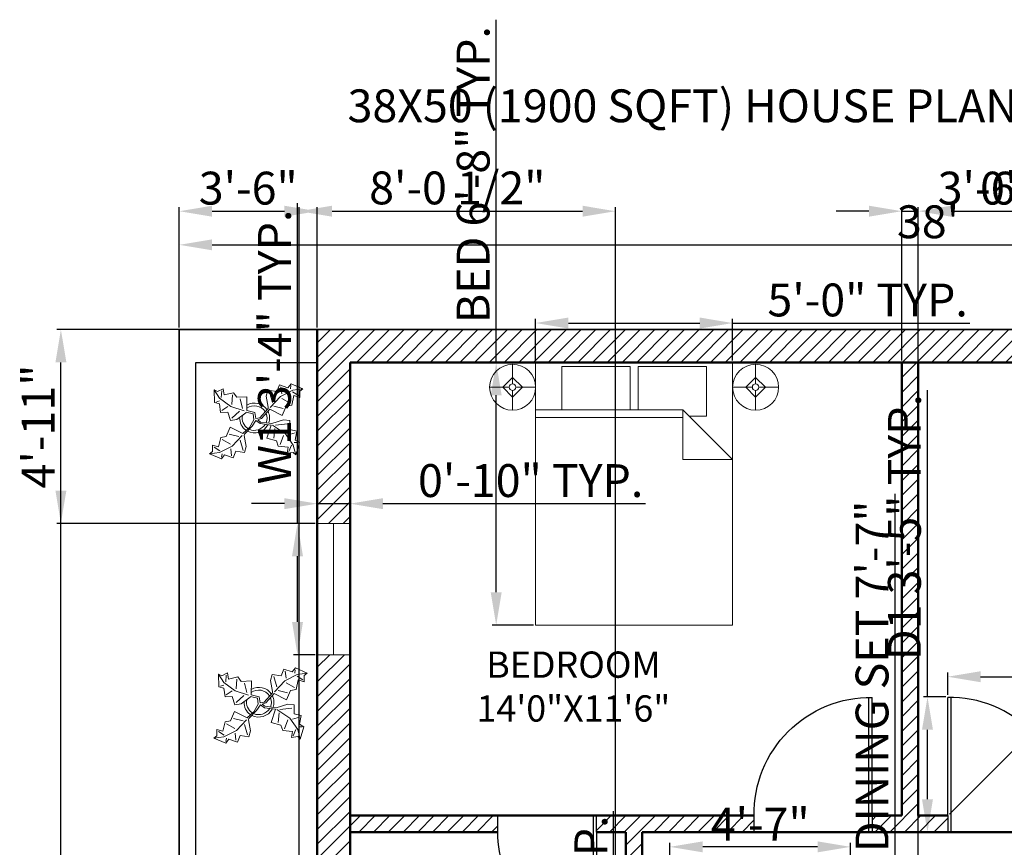
# Model space of a CAD drawing. Units: inches. Extents: x 2206 to 2843, y 1750 to 2489.
# Tile 6 of 8: x 2206 to 2506, y 2237 to 2489. Entities that reach past the tile are written whole.
import ezdxf

# ---------------------------------------------------------------- set-up
doc = ezdxf.new("R2010")
doc.units = ezdxf.units.IN
for name, color, linetype, lineweight in [('A-ANNO-DIMS', 2, 'Continuous', 18), ('A-ANNO-TEXT', 7, 'Continuous', 25), ('A-AREA-IDEN', 7, 'Continuous', 18), ('A-DOOR', 3, 'Continuous', 25), ('A-FURN', 21, 'Continuous', 18), ('A-GLAZ', 4, 'Continuous', 18), ('A-WALL', 7, 'Continuous', 50), ('A-WALL-PATT', 252, 'Continuous', 13), ('C-PROP', 7, 'Continuous', 35), ('L-PLNT', 92, 'Continuous', 18), ('L-SITE-WALL', 8, 'Continuous', 25)]:
    doc.layers.add(name, color=color, linetype=linetype, lineweight=lineweight)
doc.styles.get("Standard").update_dxf_attribs({"font": 'arial.ttf'})
doc.dimstyles.new('ISO-25', dxfattribs={"dimtxt": 10, "dimasz": 10, "dimexe": 1.25, "dimexo": 0.625, "dimtad": 1, "dimdec": 1, "dimlunit": 3, "dimtxsty": 'Standard', "dimcen": 2.5, "dimadec": 0, "dimazin": 0, "dimtfac": 1, "dimtdec": 1, "dimtmove": 0, "dimatfit": 3, "dimfxl": 1, "dimarcsym": 0})

# ---------------------------------------------------------------- blocks, each defined once
blk = doc.blocks.new('Plant - Rubber or Philodendron')
for p, q in [((-14.8639, 10.7964), (-12.6195, 11.8975)), ((-12.6195, 11.8975), (-12.1909, 9.4345)), ((8.8871, 10.7908), (9.9809, 13.4933)), ((9.9809, 13.4933), (13.3837, 12.301)), ((10.5828, 12.6946), (10.8893, 9.7953)), ((13.3837, 12.301), (14.68, 13.9039)), ((14.5816, 13.2037), (14.3848, 11.8033)), ((14.68, 13.9039), (19.3848, 11.8146)), ((-16.2005, 11.4774), (-13.9899, 8.1064)), ((-16.2005, 11.4774), (-14.8639, 10.7964)), ((-16.0159, 6.3329), (-16.2005, 11.4774)), ((-13.9899, 8.1064), (-9.5434, 4.7185)), ((-13.3174, 8.325), (-13.0735, 11.0065)), ((-12.1909, 9.4345), (-8.3829, 10.3)), ((-8.8369, 9.409), (-9.0894, 5.6095)), ((-8.3829, 10.3), (-7.0549, 8.501)), ((-7.0549, 8.501), (-3.0284, 8.6941)), ((-3.0284, 8.6941), (-3.0709, 3.1041)), ((4.6914, 8.8812), (5.3859, 11.2828)), ((4.6914, 8.8812), (5.5014, 4.4831)), ((5.3859, 11.2828), (8.8871, 10.7908)), ((5.9878, 10.4842), (7.1971, 6.3869)), ((10.3916, 8.7942), (6.2847, 4.4028)), ((15.3859, 11.3055), (10.3916, 8.7942)), ((14.2977, 6.1031), (10.9934, 7.9956)), ((15.7909, 9.1065), (14.8995, 5.3044)), ((15.2875, 10.6053), (17.5907, 9.2105)), ((19.3848, 11.8146), (15.3859, 11.3055)), ((18.1925, 8.4119), (15.7909, 9.1065)), ((19.3848, 11.8146), (18.1868, 10.9119)), ((18.1868, 10.9119), (18.1925, 8.4119)), ((-14.0069, 5.8704), (-16.0159, 6.3329)), ((-15.3434, 6.5514), (-13.9984, 6.9884)), ((-13.5868, 2.2894), (-14.0069, 5.8704)), ((-13.1329, 3.1804), (-10.6614, 4.727)), ((-9.5434, 4.7185), (-4.1917, 2.9888)), ((-4.8529, 4.012), (-5.7184, 7.82)), ((5.4346, 3.9146), (5.5014, 4.4831)), ((7.7005, 4.8881), (11.5025, 3.9967)), ((12.7005, 4.8994), (11.1089, 1.1958)), ((14.8995, 5.3044), (12.7005, 4.8994)), ((-10.6784, 2.491), (-13.5868, 2.2894)), ((-9.5858, -0.8715), (-10.6784, 2.491)), ((-9.1318, 0.0195), (-5.9793, 2.9025)), ((-7.1228, -0.443), (-3.5248, 2.2131)), ((-3.5248, 2.2131), (-3.3011, 2.4355)), ((-3.3011, 2.4355), (-0.5306, 1.7947)), ((-3.0709, 3.1041), (0.0797, 2.3163)), ((-0.5306, 1.7947), (-0.2255, -0.5527)), ((-0.5306, 1.7947), (-0.5306, 1.7947)), ((0.0797, 2.3163), (0.4866, -0.031)), ((0.4866, -0.031), (2.1141, 0.2298)), ((2.1141, 0.2298), (5.4346, 3.9146)), ((6.1032, 3.6844), (2.8262, -0.031)), ((11.1089, 1.1958), (6.1032, 3.6844)), ((-11.3237, -7.2629), (-9.7321, -3.5593)), ((-9.7321, -3.5593), (-4.7264, -6.0479)), ((-7.1228, -0.443), (-9.5858, -0.8715)), ((-2.019, -3.6148), (-4.7264, -6.0479)), ((-4.0579, -6.2781), (-0.9375, -3.1608)), ((-2.019, -3.6148), (-0.2255, -0.5527)), ((-0.9375, -3.1608), (0.5883, -0.8135)), ((0.5883, -0.8135), (2.2447, -2.0916)), ((2.8262, -0.031), (1.3003, -0.5527)), ((1.3003, -0.5527), (2.4193, -1.4655)), ((2.2447, -2.0916), (6.7108, -2.6626)), ((2.4193, -1.4655), (6.895, -2.1175)), ((4.943, -7.9659), (6.7108, -2.6626)), ((11.6605, -0.5413), (6.895, -2.1175)), ((12.3677, -6.1981), (7.219, -2.6772)), ((8.3544, -2.7453), (13.1973, -2.1704)), ((11.6605, -0.5413), (14.1354, -0.8948)), ((14.1354, -0.8948), (14.1354, -4.4304)), ((-14.4141, -11.4699), (-13.5228, -7.6679)), ((-13.5228, -7.6679), (-11.3237, -7.2629)), ((-6.3237, -7.2516), (-10.1257, -6.3602)), ((-9.0148, -11.1577), (-4.9047, -6.8122)), ((-4.1246, -6.8466), (-4.0579, -6.2781)), ((-3.3146, -11.2447), (-4.1246, -6.8466)), ((8.125, -4.0768), (7.7715, -7.9659)), ((10.2463, -10.4408), (11.6605, -6.9053)), ((15.5496, -10.7943), (12.3677, -6.1981)), ((16.2567, -5.8446), (13.4283, -6.5517)), ((14.1354, -4.4304), (16.9638, -5.1375)), ((16.9638, -5.1375), (16.2567, -8.673)), ((-16.8157, -10.7754), (-14.4141, -11.4699)), ((-16.8101, -13.2754), (-16.8157, -10.7754)), ((-13.9107, -12.9688), (-16.2139, -11.574)), ((-14.0091, -13.669), (-9.0148, -11.1577)), ((-12.921, -8.4665), (-9.6166, -10.359)), ((-4.611, -12.8477), (-5.8203, -8.7504)), ((-3.3146, -11.2447), (-4.0092, -13.6463)), ((8.8321, -9.0266), (4.943, -7.9659)), ((9.5392, -11.1479), (8.8321, -9.0266)), ((13.4283, -11.5015), (9.5392, -11.1479)), ((13.0748, -13.9763), (13.4283, -11.5015)), ((14.8425, -10.7943), (13.7819, -13.2692)), ((16.6103, -14.6834), (15.5496, -10.7943)), ((17.3174, -9.7337), (15.9032, -9.7337)), ((16.2567, -8.673), (18.0245, -9.7337)), ((18.0245, -9.7337), (16.6103, -14.6834)), ((-18.008, -14.1781), (-16.8101, -13.2754)), ((-18.008, -14.1781), (-14.0091, -13.669)), ((-13.3032, -16.2674), (-18.008, -14.1781)), ((-12.0069, -14.6645), (-13.3032, -16.2674)), ((-13.2048, -15.5672), (-13.008, -14.1668)), ((-8.6042, -15.8568), (-12.0069, -14.6645)), ((-9.206, -15.0581), (-9.5126, -12.1588)), ((-7.5103, -13.1543), (-8.6042, -15.8568)), ((-4.0092, -13.6463), (-7.5103, -13.1543)), ((15.5496, -13.6228), (13.0748, -13.9763)), ((16.6103, -14.6834), (15.5496, -13.6228))]:
    blk.add_line(p, q)
for centre, radius, start, end in [((0, 0), 6.1275, 34.37569, 120.1028), ((-0.0601, -0.2075), 5.2461, 33.82192, 124.9414), ((0.0308, 0.1664), 6, 178.6147, 235.1169), ((0.0308, 0.1664), 5, 168.1647, 238.6725), ((-0.2664, 0.1682), 5.2775, 338.4094, 20.03007), ((-0.098, 0.1364), 6.1288, 341.2017, 26.09184), ((-0.0234, 0.3825), 6.1492, 242.5812, 331.2714), ((-0.1102, 0.4886), 5.2883, 247.3711, 327.472)]:
    blk.add_arc(centre, radius, start, end)
blk = doc.blocks.new('Bed - Queen')
for p, q in [((0, -80.00003), (0, 0)), ((0, 0), (59.99999, 0)), ((59.99999, 0), (59.99999, -80.00003)), ((7.99999, -1.2), (28.79998, -1.2)), ((7.99999, -14.4), (7.99999, -1.2)), ((28.79998, -1.2), (28.79998, -14.4)), ((31.19999, -1.2), (51.99999, -1.2)), ((31.19999, -14.4), (31.19999, -1.2)), ((51.99999, -1.2), (51.99999, -16.4)), ((0, -14.4), (44.8, -14.4)), ((59.99999, -29.6), (44.8, -14.4)), ((44.8, -14.4), (44.8, -29.6)), ((44.8, -16.8), (0, -16.8)), ((51.99999, -16.4), (46.79936, -16.4)), ((44.8, -29.6), (59.99999, -29.6)), ((59.99999, -80.00003), (0, -80.00003))]:
    blk.add_line(p, q)
blk = doc.blocks.new('Lamp - Table')
for p, q in [((0, 7), (0, 1)), ((0, 3), (-3, 0)), ((3, 0), (0, 3)), ((-1, 0), (-7, 0)), ((-3, 0), (0, -3)), ((0, -3), (3, 0)), ((1, 0), (7, 0)), ((0, -1), (0, -7))]:
    blk.add_line(p, q)
for radius in [7, 1]:
    blk.add_circle((0, 0), radius)
blk = doc.blocks.new('*D14')
at = {"layer": 'A-ANNO-DIMS', "color": 0, "lineweight": -2, "transparency": 16777216}
for p, q in [((2254.58, 2395.52), (2254.58, 2421.96)), ((2264.58, 2420.71), (2700.58, 2420.71)), ((2710.58, 2395.52), (2710.58, 2421.96))]:
    blk.add_line(p, q, dxfattribs=at)
at = {"layer": 'A-ANNO-DIMS', "color": 0, "transparency": 16777216}
for points in [[(2264.58, 2422.38), (2264.58, 2419.04), (2254.58, 2420.71)], [(2700.58, 2422.38), (2700.58, 2419.04), (2710.58, 2420.71)]]:
    blk.add_solid(points, dxfattribs=at)
at = {"layer": 'Defpoints', "color": 0, "transparency": 16777216}
for p in [(2710.58, 2420.71), (2254.58, 2394.9), (2710.58, 2394.9)]:
    blk.add_point(p, dxfattribs=at)
at = {"layer": 'A-ANNO-DIMS', "color": 0, "transparency": 16777216, "insert": (2482.58, 2426.44), "char_height": 10, "attachment_point": 5}
blk.add_mtext("38'", dxfattribs=at)
blk = doc.blocks.new('WIN-40IN')
for p, q in [((10, 40), (0, 40)), ((5, 40), (5, 0)), ((10, 0), (0, 0))]:
    blk.add_line(p, q)
blk = doc.blocks.new('DOOR-SWING-36IN')
for p, q in [((0, 5), (0, 41)), ((1, 0), (1, 41)), ((0, 5), (0, 0)), ((36, 5), (36, 0))]:
    blk.add_line(p, q)
blk.add_arc((0.5, 5.5), 35.5, 359.1931, 90.8069)
blk = doc.blocks.new('DOOR-SWING-30IN')
for p, q in [((29, 0), (29, 35)), ((30, 5), (30, 35))]:
    blk.add_line(p, q)
blk.add_arc((29.5, 5.5), 29.5, 89.029, 180.971)
blk = doc.blocks.new('*D31')
at = {"layer": 'A-ANNO-DIMS', "color": 0, "lineweight": -2, "transparency": 16777216}
for p, q in [((2351.08, 2384.9), (2351.08, 2489.27)), ((2362.45, 2384.9), (2349.83, 2384.9)), ((2351.08, 2314.9), (2351.08, 2374.9)), ((2362.45, 2304.9), (2349.83, 2304.9))]:
    blk.add_line(p, q, dxfattribs=at)
at = {"layer": 'A-ANNO-DIMS', "color": 0, "transparency": 16777216}
for points in [[(2349.41, 2374.9), (2352.75, 2374.9), (2351.08, 2384.9)], [(2349.41, 2314.9), (2352.75, 2314.9), (2351.08, 2304.9)]]:
    blk.add_solid(points, dxfattribs=at)
at = {"layer": 'Defpoints', "color": 0, "transparency": 16777216}
for p in [(2351.08, 2384.9), (2363.08, 2384.9), (2363.08, 2304.9)]:
    blk.add_point(p, dxfattribs=at)
at = {"layer": 'A-ANNO-DIMS', "color": 0, "transparency": 16777216, "insert": (2345.35, 2442.08), "char_height": 10, "attachment_point": 5, "rotation": 90}
blk.add_mtext('BED 6\'-8" TYP.', dxfattribs=at)
blk = doc.blocks.new('*D32')
at = {"layer": 'A-ANNO-DIMS', "color": 0, "lineweight": -2, "transparency": 16777216}
for p, q in [((2363.08, 2385.52), (2363.08, 2398.15)), ((2373.08, 2396.9), (2413.08, 2396.9)), ((2423.08, 2385.52), (2423.08, 2398.15)), ((2423.08, 2396.9), (2495.28, 2396.9))]:
    blk.add_line(p, q, dxfattribs=at)
at = {"layer": 'A-ANNO-DIMS', "color": 0, "transparency": 16777216}
for points in [[(2373.08, 2398.57), (2373.08, 2395.23), (2363.08, 2396.9)], [(2413.08, 2398.57), (2413.08, 2395.23), (2423.08, 2396.9)]]:
    blk.add_solid(points, dxfattribs=at)
at = {"layer": 'Defpoints', "color": 0, "transparency": 16777216}
for p in [(2423.08, 2396.9), (2363.08, 2384.9), (2423.08, 2384.9)]:
    blk.add_point(p, dxfattribs=at)
at = {"layer": 'A-ANNO-DIMS', "color": 0, "transparency": 16777216, "insert": (2464.18, 2402.63), "char_height": 10, "attachment_point": 5}
blk.add_mtext('5\'-0" TYP.', dxfattribs=at)
blk = doc.blocks.new('*D35')
at = {"layer": 'A-ANNO-DIMS', "color": 0, "lineweight": -2, "transparency": 16777216}
for p, q in [((2290.58, 2335.9), (2290.58, 2433.35)), ((2295.95, 2335.9), (2289.33, 2335.9)), ((2290.58, 2305.9), (2290.58, 2325.9)), ((2295.95, 2295.9), (2289.33, 2295.9))]:
    blk.add_line(p, q, dxfattribs=at)
at = {"layer": 'A-ANNO-DIMS', "color": 0, "transparency": 16777216}
for points in [[(2288.91, 2325.9), (2292.25, 2325.9), (2290.58, 2335.9)], [(2288.91, 2305.9), (2292.25, 2305.9), (2290.58, 2295.9)]]:
    blk.add_solid(points, dxfattribs=at)
at = {"layer": 'Defpoints', "color": 0, "transparency": 16777216}
for p in [(2290.58, 2335.9), (2296.58, 2335.9), (2296.58, 2295.9)]:
    blk.add_point(p, dxfattribs=at)
at = {"layer": 'A-ANNO-DIMS', "color": 0, "transparency": 16777216, "insert": (2284.85, 2389.62), "char_height": 10, "attachment_point": 5, "rotation": 90}
blk.add_mtext('W1 3\'-4" TYP.', dxfattribs=at)
blk = doc.blocks.new('*D36')
at = {"layer": 'A-ANNO-DIMS', "color": 0, "lineweight": -2, "transparency": 16777216}
for p, q in [((2286.58, 2341.9), (2276.58, 2341.9)), ((2296.58, 2336.52), (2296.58, 2343.15)), ((2296.58, 2341.9), (2306.58, 2341.9)), ((2306.58, 2336.52), (2306.58, 2343.15)), ((2316.58, 2341.9), (2396.55, 2341.9))]:
    blk.add_line(p, q, dxfattribs=at)
at = {"layer": 'A-ANNO-DIMS', "color": 0, "transparency": 16777216}
for points in [[(2286.58, 2343.57), (2286.58, 2340.23), (2296.58, 2341.9)], [(2316.58, 2343.57), (2316.58, 2340.23), (2306.58, 2341.9)]]:
    blk.add_solid(points, dxfattribs=at)
at = {"layer": 'Defpoints', "color": 0, "transparency": 16777216}
for p in [(2306.58, 2341.9), (2296.58, 2335.9), (2306.58, 2335.9)]:
    blk.add_point(p, dxfattribs=at)
at = {"layer": 'A-ANNO-DIMS', "color": 0, "transparency": 16777216, "insert": (2361.57, 2347.63), "char_height": 10, "attachment_point": 5}
blk.add_mtext('0\'-10" TYP.', dxfattribs=at)
blk = doc.blocks.new('*D41')
at = {"layer": 'A-ANNO-DIMS', "color": 0, "lineweight": -2, "transparency": 16777216}
for p, q in [((2482.41, 2283.03), (2482.41, 2376.48)), ((2487.95, 2283.03), (2481.16, 2283.03)), ((2482.41, 2251.9), (2482.41, 2273.03)), ((2487.95, 2241.9), (2481.16, 2241.9))]:
    blk.add_line(p, q, dxfattribs=at)
at = {"layer": 'A-ANNO-DIMS', "color": 0, "transparency": 16777216}
for points in [[(2480.74, 2273.03), (2484.08, 2273.03), (2482.41, 2283.03)], [(2480.74, 2251.9), (2484.08, 2251.9), (2482.41, 2241.9)]]:
    blk.add_solid(points, dxfattribs=at)
at = {"layer": 'Defpoints', "color": 0, "transparency": 16777216}
for p in [(2482.41, 2283.03), (2488.58, 2283.03), (2488.58, 2241.9)]:
    blk.add_point(p, dxfattribs=at)
at = {"layer": 'A-ANNO-DIMS', "color": 0, "transparency": 16777216, "insert": (2476.68, 2334.76), "char_height": 10, "attachment_point": 5, "rotation": 90}
blk.add_mtext('D1 3\'-5" TYP.', dxfattribs=at)
blk = doc.blocks.new('*D42')
at = {"layer": 'A-ANNO-DIMS', "color": 0, "lineweight": -2, "transparency": 16777216}
for p, q in [((2488.58, 2283.66), (2488.58, 2290.45)), ((2498.58, 2289.2), (2514.71, 2289.2)), ((2524.71, 2283.66), (2524.71, 2290.45)), ((2524.71, 2289.2), (2596.91, 2289.2))]:
    blk.add_line(p, q, dxfattribs=at)
at = {"layer": 'A-ANNO-DIMS', "color": 0, "transparency": 16777216}
for points in [[(2498.58, 2290.87), (2498.58, 2287.54), (2488.58, 2289.2)], [(2514.71, 2290.87), (2514.71, 2287.54), (2524.71, 2289.2)]]:
    blk.add_solid(points, dxfattribs=at)
at = {"layer": 'Defpoints', "color": 0, "transparency": 16777216}
for p in [(2524.71, 2289.2), (2488.58, 2283.03), (2524.71, 2283.03)]:
    blk.add_point(p, dxfattribs=at)
at = {"layer": 'A-ANNO-DIMS', "color": 0, "transparency": 16777216, "insert": (2565.81, 2294.94), "char_height": 10, "attachment_point": 5}
blk.add_mtext('3\'-0" TYP.', dxfattribs=at)
blk = doc.blocks.new('*D43')
at = {"layer": 'A-ANNO-DIMS', "color": 0, "lineweight": -2, "transparency": 16777216}
for p, q in [((2386.85, 2147.03), (2386.85, 2248.25)), ((2382.2, 2147.03), (2388.1, 2147.03)), ((2386.85, 2121.9), (2386.85, 2137.03)), ((2382.2, 2111.9), (2388.1, 2111.9))]:
    blk.add_line(p, q, dxfattribs=at)
at = {"layer": 'A-ANNO-DIMS', "color": 0, "transparency": 16777216}
for points in [[(2385.18, 2137.03), (2388.52, 2137.03), (2386.85, 2147.03)], [(2385.18, 2121.9), (2388.52, 2121.9), (2386.85, 2111.9)]]:
    blk.add_solid(points, dxfattribs=at)
at = {"layer": 'Defpoints', "color": 0, "transparency": 16777216}
for p in [(2381.58, 2147.03), (2386.85, 2147.03), (2381.58, 2111.9)]:
    blk.add_point(p, dxfattribs=at)
at = {"layer": 'A-ANNO-DIMS', "color": 0, "transparency": 16777216, "insert": (2381.2, 2202.64), "char_height": 10, "attachment_point": 5, "rotation": 90}
blk.add_mtext('D2 2\'-11" TYP.', dxfattribs=at)
blk = doc.blocks.new('*D47')
at = {"layer": 'A-ANNO-DIMS', "color": 0, "lineweight": -2, "transparency": 16777216}
for p, q in [((2472.62, 2223.74), (2472.62, 2344.9)), ((2459.59, 2223.74), (2473.87, 2223.74)), ((2472.62, 2142.74), (2472.62, 2213.74)), ((2459.59, 2132.74), (2473.87, 2132.74))]:
    blk.add_line(p, q, dxfattribs=at)
at = {"layer": 'A-ANNO-DIMS', "color": 0, "transparency": 16777216}
for points in [[(2470.95, 2213.74), (2474.28, 2213.74), (2472.62, 2223.74)], [(2470.95, 2142.74), (2474.28, 2142.74), (2472.62, 2132.74)]]:
    blk.add_solid(points, dxfattribs=at)
at = {"layer": 'Defpoints', "color": 0, "transparency": 16777216}
for p in [(2458.97, 2223.74), (2472.62, 2223.74), (2458.97, 2132.74)]:
    blk.add_point(p, dxfattribs=at)
at = {"layer": 'A-ANNO-DIMS', "color": 0, "transparency": 16777216, "insert": (2466.82, 2289.32), "char_height": 10, "attachment_point": 5, "rotation": 90}
blk.add_mtext('DINING SET 7\'-7"', dxfattribs=at)
blk = doc.blocks.new('*D48')
at = {"layer": 'A-ANNO-DIMS', "color": 0, "lineweight": -2, "transparency": 16777216}
for p, q in [((2403.97, 2224.37), (2403.97, 2238.64)), ((2448.97, 2237.39), (2413.97, 2237.39)), ((2458.97, 2224.37), (2458.97, 2238.64))]:
    blk.add_line(p, q, dxfattribs=at)
at = {"layer": 'A-ANNO-DIMS', "color": 0, "transparency": 16777216}
for points in [[(2413.97, 2239.06), (2413.97, 2235.73), (2403.97, 2237.39)], [(2448.97, 2239.06), (2448.97, 2235.73), (2458.97, 2237.39)]]:
    blk.add_solid(points, dxfattribs=at)
at = {"layer": 'Defpoints', "color": 0, "transparency": 16777216}
for p in [(2403.97, 2237.39), (2403.97, 2223.74), (2458.97, 2223.74)]:
    blk.add_point(p, dxfattribs=at)
at = {"layer": 'A-ANNO-DIMS', "color": 0, "transparency": 16777216, "insert": (2431.47, 2243.02), "char_height": 10, "attachment_point": 5}
blk.add_mtext('4\'-7"', dxfattribs=at)
blk = doc.blocks.new('*D57')
at = {"layer": 'A-ANNO-DIMS', "color": 0, "lineweight": -2, "transparency": 16777216}
for p, q in [((2254.58, 2395.52), (2254.58, 2432.2)), ((2296.58, 2395.52), (2296.58, 2432.2)), ((2264.58, 2430.95), (2286.58, 2430.95))]:
    blk.add_line(p, q, dxfattribs=at)
at = {"layer": 'A-ANNO-DIMS', "color": 0, "transparency": 16777216}
for points in [[(2264.58, 2432.62), (2264.58, 2429.28), (2254.58, 2430.95)], [(2286.58, 2432.62), (2286.58, 2429.28), (2296.58, 2430.95)]]:
    blk.add_solid(points, dxfattribs=at)
at = {"layer": 'Defpoints', "color": 0, "transparency": 16777216}
for p in [(2296.58, 2430.95), (2254.58, 2394.9), (2296.58, 2394.9)]:
    blk.add_point(p, dxfattribs=at)
at = {"layer": 'A-ANNO-DIMS', "color": 0, "transparency": 16777216, "insert": (2275.58, 2436.68), "char_height": 10, "attachment_point": 5}
blk.add_mtext('3\'-6"', dxfattribs=at)
blk = doc.blocks.new('*D58')
at = {"layer": 'A-ANNO-DIMS', "color": 0, "lineweight": -2, "transparency": 16777216}
for p, q in [((2295.95, 2394.9), (2217.28, 2394.9)), ((2218.53, 1991.9), (2218.53, 2384.9)), ((2295.95, 1981.9), (2217.28, 1981.9))]:
    blk.add_line(p, q, dxfattribs=at)
at = {"layer": 'A-ANNO-DIMS', "color": 0, "transparency": 16777216}
for points in [[(2216.86, 2384.9), (2220.2, 2384.9), (2218.53, 2394.9)], [(2216.86, 1991.9), (2220.2, 1991.9), (2218.53, 1981.9)]]:
    blk.add_solid(points, dxfattribs=at)
at = {"layer": 'Defpoints', "color": 0, "transparency": 16777216}
for p in [(2218.53, 2394.9), (2296.58, 2394.9), (2296.58, 1981.9)]:
    blk.add_point(p, dxfattribs=at)
at = {"layer": 'A-ANNO-DIMS', "color": 0, "transparency": 16777216, "insert": (2212.8, 2188.4), "char_height": 10, "attachment_point": 5, "rotation": 90}
blk.add_mtext('34\'-5"', dxfattribs=at)
blk = doc.blocks.new('*D61')
at = {"layer": 'A-ANNO-DIMS', "color": 0, "lineweight": -2, "transparency": 16777216}
for p, q in [((2479.58, 2100.52), (2479.58, 2432.2)), ((2521.58, 2100.52), (2521.58, 2432.2)), ((2489.58, 2430.95), (2511.58, 2430.95))]:
    blk.add_line(p, q, dxfattribs=at)
at = {"layer": 'A-ANNO-DIMS', "color": 0, "transparency": 16777216}
for points in [[(2489.58, 2432.62), (2489.58, 2429.28), (2479.58, 2430.95)], [(2511.58, 2432.62), (2511.58, 2429.28), (2521.58, 2430.95)]]:
    blk.add_solid(points, dxfattribs=at)
at = {"layer": 'Defpoints', "color": 0, "transparency": 16777216}
for p in [(2521.58, 2430.95), (2479.58, 2099.9), (2521.58, 2099.9)]:
    blk.add_point(p, dxfattribs=at)
at = {"layer": 'A-ANNO-DIMS', "color": 0, "transparency": 16777216, "insert": (2500.58, 2436.68), "char_height": 10, "attachment_point": 5}
blk.add_mtext('3\'-6"', dxfattribs=at)
blk = doc.blocks.new('*D65')
at = {"layer": 'A-ANNO-DIMS', "color": 0, "lineweight": -2, "transparency": 16777216}
for p, q in [((2474.58, 2385.52), (2474.58, 2432.2)), ((2479.58, 2385.52), (2479.58, 2432.2)), ((2464.58, 2430.95), (2454.58, 2430.95)), ((2474.58, 2430.95), (2479.58, 2430.95)), ((2489.58, 2430.95), (2527.41, 2430.95))]:
    blk.add_line(p, q, dxfattribs=at)
at = {"layer": 'A-ANNO-DIMS', "color": 0, "transparency": 16777216}
for points in [[(2464.58, 2432.62), (2464.58, 2429.28), (2474.58, 2430.95)], [(2489.58, 2432.62), (2489.58, 2429.28), (2479.58, 2430.95)]]:
    blk.add_solid(points, dxfattribs=at)
at = {"layer": 'Defpoints', "color": 0, "transparency": 16777216}
for p in [(2479.58, 2430.95), (2474.58, 2384.9), (2479.58, 2384.9)]:
    blk.add_point(p, dxfattribs=at)
at = {"layer": 'A-ANNO-DIMS', "color": 0, "transparency": 16777216, "insert": (2513.5, 2436.68), "char_height": 10, "attachment_point": 5}
blk.add_mtext('0\'-5"', dxfattribs=at)
blk = doc.blocks.new('*D66')
at = {"layer": 'A-ANNO-DIMS', "color": 0, "lineweight": -2, "transparency": 16777216}
for p, q in [((2295.95, 2394.9), (2217.28, 2394.9)), ((2218.53, 2345.9), (2218.53, 2384.9)), ((2295.95, 2335.9), (2217.28, 2335.9))]:
    blk.add_line(p, q, dxfattribs=at)
at = {"layer": 'A-ANNO-DIMS', "color": 0, "transparency": 16777216}
for points in [[(2216.86, 2384.9), (2220.2, 2384.9), (2218.53, 2394.9)], [(2216.86, 2345.9), (2220.2, 2345.9), (2218.53, 2335.9)]]:
    blk.add_solid(points, dxfattribs=at)
at = {"layer": 'Defpoints', "color": 0, "transparency": 16777216}
for p in [(2218.53, 2394.9), (2296.58, 2394.9), (2296.58, 2335.9)]:
    blk.add_point(p, dxfattribs=at)
at = {"layer": 'A-ANNO-DIMS', "color": 0, "transparency": 16777216, "insert": (2212.88, 2365.4), "char_height": 10, "attachment_point": 5, "rotation": 90}
blk.add_mtext('4\'-11"', dxfattribs=at)
blk = doc.blocks.new('*D72')
at = {"layer": 'A-ANNO-DIMS', "color": 0, "lineweight": -2, "transparency": 16777216}
for p, q in [((2291.11, 1795.52), (2291.11, 2432.2)), ((2387.37, 1795.52), (2387.37, 2432.2)), ((2301.11, 2430.95), (2377.37, 2430.95))]:
    blk.add_line(p, q, dxfattribs=at)
at = {"layer": 'A-ANNO-DIMS', "color": 0, "transparency": 16777216}
for points in [[(2301.11, 2432.62), (2301.11, 2429.28), (2291.11, 2430.95)], [(2377.37, 2432.62), (2377.37, 2429.28), (2387.37, 2430.95)]]:
    blk.add_solid(points, dxfattribs=at)
at = {"layer": 'Defpoints', "color": 0, "transparency": 16777216}
for p in [(2387.37, 2430.95), (2291.11, 1794.9), (2387.37, 1794.9)]:
    blk.add_point(p, dxfattribs=at)
at = {"layer": 'A-ANNO-DIMS', "color": 0, "transparency": 16777216, "insert": (2339.24, 2436.74), "char_height": 10, "attachment_point": 5}
blk.add_mtext('8\'-0 1/2"', dxfattribs=at)
blk = doc.blocks.new('*D83')
at = {"layer": 'A-ANNO-DIMS', "color": 0, "lineweight": -2, "transparency": 16777216}
for p, q in [((2592.06, 2350.38), (2521.26, 2279.57)), ((2489.08, 2247.4), (2514.18, 2272.5))]:
    blk.add_line(p, q, dxfattribs=at)
at = {"layer": 'A-ANNO-DIMS', "color": 0, "transparency": 16777216}
blk.add_solid([(2520.08, 2280.75), (2522.43, 2278.4), (2514.18, 2272.5)], dxfattribs=at)
at = {"layer": 'Defpoints', "color": 0, "transparency": 16777216}
for p in [(2514.18, 2272.5), (2489.08, 2247.4)]:
    blk.add_point(p, dxfattribs=at)
at = {"layer": 'A-ANNO-DIMS', "color": 0, "transparency": 16777216, "insert": (2556.1, 2322.61), "char_height": 10, "attachment_point": 5, "rotation": 44.9995}
blk.add_mtext('2X R2\'-11 1/2"', dxfattribs=at)

msp = doc.modelspace()

# ---------------------------------------------------------------- hatches: boundary and pattern name
at = {"layer": 'A-WALL-PATT'}
h = msp.add_hatch(dxfattribs=at)
h.set_pattern_fill('ANSI31', color=256)
h.paths.add_polyline_path([(2710.58, 2394.9), (2296.58, 2394.9), (2296.58, 2335.9), (2306.58, 2335.9), (2306.58, 2384.9), (2479.58, 2384.9), (2652.58, 2384.9), (2700.58, 2384.9), (2700.58, 2300.9), (2690.58, 2300.9), (2690.58, 2290.9), (2710.58, 2290.9)])
h.paths.add_polyline_path([(2306.58, 2295.9), (2296.58, 2295.9), (2296.58, 2225.9), (2306.58, 2225.9), (2306.58, 2241.9)])
h.paths.add_polyline_path([(2306.58, 2111.9), (2306.58, 2132.9), (2296.58, 2132.9), (2296.58, 2071.9), (2306.58, 2071.9)])
h.paths.add_polyline_path([(2306.58, 2197.9), (2296.58, 2197.9), (2296.58, 2160.9), (2306.58, 2160.9), (2306.58, 2176.9)])
h.paths.add_polyline_path([(2370.58, 1991.9), (2306.58, 1991.9), (2306.58, 2031.9), (2296.58, 2031.9), (2296.58, 1981.9), (2370.58, 1981.9)])
h.paths.add_polyline_path([(2479.58, 2066.9), (2474.58, 2066.9), (2474.58, 1991.9), (2410.58, 1991.9), (2410.58, 1981.9), (2479.58, 1981.9)])
h.paths.add_polyline_path([(2539.58, 1943.9), (2479.58, 1943.9), (2479.58, 1944.9), (2469.58, 1944.9), (2469.58, 1933.9), (2539.58, 1933.9)])
h.paths.add_polyline_path([(2657.58, 1997.9), (2647.58, 1997.9), (2647.58, 1943.9), (2647.58, 1918.9), (2657.58, 1918.9)])
h.paths.add_polyline_path([(2647.58, 1943.9), (2587.58, 1943.9), (2587.58, 1933.9), (2647.58, 1933.9)])
h.paths.add_polyline_path([(2657.58, 2158.4), (2647.58, 2158.4), (2647.58, 2104.9), (2647.58, 2045.9), (2657.58, 2045.9)])
h.paths.add_polyline_path([(2657.58, 2204.89), (2647.58, 2204.89), (2647.58, 2188.4), (2657.58, 2188.4)])
h.paths.add_polyline_path([(2657.58, 2246.9), (2647.58, 2246.9), (2647.58, 2234.9), (2657.58, 2234.9)])
h.paths.add_polyline_path([(2662.58, 2300.9), (2652.58, 2300.9), (2652.58, 2346.22), (2647.58, 2346.22), (2647.58, 2290.9), (2662.58, 2290.9)])
h.paths.add_polyline_path([(2647.58, 2246.9), (2524.58, 2246.9), (2524.58, 2241.9), (2647.58, 2241.9)])
h.paths.add_polyline_path([(2351.58, 2246.9), (2306.58, 2246.9), (2306.58, 2241.9), (2351.58, 2241.9)])
h.paths.add_polyline_path([(2429.58, 2246.9), (2381.58, 2246.9), (2381.58, 2241.9), (2390.58, 2241.9), (2390.58, 2181.9), (2306.58, 2181.9), (2306.58, 2176.9), (2390.58, 2176.9), (2390.58, 2116.9), (2381.58, 2116.9), (2381.58, 2111.9), (2474.58, 2111.9), (2474.58, 2102.9), (2479.58, 2102.9), (2479.58, 2104.9), (2479.58, 2116.9), (2395.58, 2116.9), (2395.58, 2176.9), (2395.58, 2241.9), (2429.58, 2241.9)])
h.paths.add_polyline_path([(2479.58, 2384.9), (2474.58, 2384.9), (2474.58, 2246.9), (2465.58, 2246.9), (2465.58, 2241.9), (2479.58, 2241.9), (2488.58, 2241.9), (2488.58, 2246.9), (2479.58, 2246.9)])
h.paths.add_polyline_path([(2657.58, 1870.9), (2647.58, 1870.9), (2647.58, 1855.9), (2511.58, 1855.9), (2511.58, 1845.9), (2657.58, 1845.9)])

# ---------------------------------------------------------------- linework, layer by layer
at = {"layer": 'A-DOOR'}
for p, q in [((2351.58, 2241.4), (2351.58, 2246.9)), ((2381.58, 2241.9), (2381.58, 2246.9))]:
    msp.add_line(p, q, dxfattribs=at)
at = {"layer": 'A-WALL'}
for p, q in [((2296.58, 1981.9), (2296.58, 2394.9)), ((2306.58, 2384.9), (2479.58, 2384.9)), ((2306.58, 2241.9), (2306.58, 2384.9)), ((2474.58, 2246.9), (2474.58, 2384.9)), ((2479.58, 2384.9), (2479.58, 2246.9)), ((2479.58, 2384.9), (2652.58, 2384.9)), ((2306.58, 2246.9), (2429.58, 2246.9)), ((2465.58, 2246.9), (2474.58, 2246.9)), ((2479.58, 2246.9), (2488.58, 2246.9)), ((2306.58, 2241.9), (2351.58, 2241.9)), ((2306.58, 2176.9), (2306.58, 2241.9)), ((2390.58, 2241.9), (2381.58, 2241.9)), ((2381.58, 2241.9), (2390.58, 2241.9)), ((2390.58, 2181.9), (2390.58, 2241.9)), ((2395.58, 2176.9), (2395.58, 2241.9)), ((2395.58, 2241.9), (2479.58, 2241.9)), ((2479.58, 2241.9), (2647.58, 2241.9))]:
    msp.add_line(p, q, dxfattribs=at)
at = {"layer": 'C-PROP'}
for p, q in [((2254.58, 2394.9), (2710.58, 2394.9)), ((2254.58, 1794.9), (2254.58, 2394.9))]:
    msp.add_line(p, q, dxfattribs=at)
at = {"layer": 'L-SITE-WALL'}
for p, q in [((2259.58, 1799.9), (2259.58, 2384.9)), ((2259.58, 2384.9), (2296.58, 2384.9))]:
    msp.add_line(p, q, dxfattribs=at)

# ---------------------------------------------------------------- block references
at = {"layer": 'A-DOOR', "extrusion": (0, 0, -1), "zscale": -1}
msp.add_blockref('DOOR-SWING-36IN', (-2465.58, 2241.9), dxfattribs=at)
at = {"layer": 'A-DOOR'}
msp.add_blockref('DOOR-SWING-36IN', (2488.58, 2241.9), dxfattribs=at)
at = {"layer": 'A-DOOR', "extrusion": (0, 0, -1), "zscale": -1, "rotation": 180}
msp.add_blockref('DOOR-SWING-30IN', (-2351.58, 2246.9), dxfattribs=at)
at = {"layer": 'A-FURN'}
for name, p in [('Lamp - Table', (2356.08, 2377.35)), ('Bed - Queen', (2363.08, 2384.9))]:
    msp.add_blockref(name, p, dxfattribs=at)
at = {"layer": 'A-FURN', "xscale": -1}
msp.add_blockref('Lamp - Table', (2430.08, 2377.35), dxfattribs=at)
at = {"layer": 'A-GLAZ'}
msp.add_blockref('WIN-40IN', (2296.58, 2295.9), dxfattribs=at)
at = {"layer": 'L-PLNT', "xscale": 0.7595985084536371, "yscale": 0.7595985084536371, "zscale": 0.7595985084536371}
for p in [(2277.49, 2367.87), (2278.82, 2281.3)]:
    msp.add_blockref('Plant - Rubber or Philodendron', p, dxfattribs=at)

# ---------------------------------------------------------------- texts
at = {"layer": 'A-ANNO-TEXT', "insert": (2305.82, 2468.04), "char_height": 10, "attachment_point": 1}
msp.add_mtext_dynamic_manual_height_columns('{\\fArial|b1|i0|c0|p34;38X50 (1900 SQFT) HOUSE PLAN - WEST FACE - FP1317}', width=488.3638, gutter_width=12.5, heights=[0], dxfattribs=at)
at = {"layer": 'A-AREA-IDEN', "insert": (2328.59, 2296.88), "char_height": 8, "attachment_point": 1}
msp.add_mtext_dynamic_manual_height_columns('\\pxqc;BEDROOM\\P14\'0"X11\'6"', width=91.9993, gutter_width=12.5, heights=[0], dxfattribs=at)

# ---------------------------------------------------------------- dimensions: what is measured, and where the dimension line sits
at = {"layer": 'A-ANNO-DIMS'}
for base, p1, p2, text, picture, middle in [((2351.08, 2384.9), (2363.08, 2304.9), (2363.08, 2384.9), 'BED <> TYP.', '*D31', (2345.35, 2442.08)), ((2290.58, 2335.9), (2296.58, 2295.9), (2296.58, 2335.9), 'W1 <> TYP.', '*D35', (2284.85, 2389.62)), ((2482.41, 2283.03), (2488.58, 2241.9), (2488.58, 2283.03), 'D1 <> TYP.', '*D41', (2476.68, 2334.76)), ((2472.62, 2223.74), (2458.97, 2132.74), (2458.97, 2223.74), 'DINING SET <>', '*D47', (2466.82, 2289.32)), ((2386.85, 2147.03), (2381.58, 2111.9), (2381.58, 2147.03), 'D2 <> TYP.', '*D43', (2381.2, 2202.64))]:
    dim = msp.add_linear_dim(base=base, p1=p1, p2=p2, angle=90, text=text, dimstyle='ISO-25', override={"dimdec": 1, "dimlfac": 1, "dimrnd": 0, "dimzin": 1, "dimdsep": 46, "dimlunit": 4, "dimfrac": 2}, dxfattribs=at)
    dim.commit()
    dim.dimension.update_dxf_attribs({"geometry": picture, "text_midpoint": middle})
for base, p1, p2, override, picture, middle in [((2387.37, 2430.95), (2291.11, 1794.9), (2387.37, 1794.9), {"dimdec": 1, "dimlfac": 1, "dimrnd": 0, "dimzin": 1, "dimdsep": 46, "dimlunit": 4, "dimfrac": 2}, '*D72', (2339.24, 2436.74)), ((2296.58, 2430.95), (2254.58, 2394.9), (2296.58, 2394.9), {"dimdec": 1, "dimlfac": 1, "dimrnd": 0, "dimzin": 1, "dimdsep": 46, "dimlunit": 4, "dimfrac": 2}, '*D57', (2275.58, 2436.68)), ((2479.58, 2430.95), (2474.58, 2384.9), (2479.58, 2384.9), {"dimdec": 1, "dimlfac": 1, "dimrnd": 0, "dimzin": 1, "dimdsep": 46, "dimlunit": 4, "dimfrac": 2}, '*D65', (2513.5, 2436.68)), ((2521.58, 2430.95), (2479.58, 2099.9), (2521.58, 2099.9), {"dimdec": 1, "dimlfac": 1, "dimrnd": 0, "dimzin": 1, "dimdsep": 46, "dimlunit": 4, "dimfrac": 2}, '*D61', (2500.58, 2436.68)), ((2710.58, 2420.71), (2254.58, 2394.9), (2710.58, 2394.9), {"dimclrd": 0, "dimclre": 0, "dimclrt": 0}, '*D14', (2482.58, 2426.44))]:
    dim = msp.add_linear_dim(base=base, p1=p1, p2=p2, dimstyle='ISO-25', override=override, dxfattribs=at)
    dim.commit()
    dim.dimension.update_dxf_attribs({"geometry": picture, "text_midpoint": middle})
for base, p1, p2, picture, middle in [((2423.08, 2396.9), (2363.08, 2384.9), (2423.08, 2384.9), '*D32', (2464.18, 2402.63)), ((2306.58, 2341.9), (2296.58, 2335.9), (2306.58, 2335.9), '*D36', (2361.57, 2347.63)), ((2524.71, 2289.2), (2488.58, 2283.03), (2524.71, 2283.03), '*D42', (2565.81, 2294.94))]:
    dim = msp.add_linear_dim(base=base, p1=p1, p2=p2, text='<> TYP.', dimstyle='ISO-25', override={"dimdec": 1, "dimlfac": 1, "dimrnd": 0, "dimzin": 1, "dimdsep": 46, "dimlunit": 4, "dimfrac": 2}, dxfattribs=at)
    dim.commit()
    dim.dimension.update_dxf_attribs({"geometry": picture, "text_midpoint": middle})
for base, p1, p2, angle, picture, middle in [((2218.53, 2394.9), (2296.58, 1981.9), (2296.58, 2394.9), 90, '*D58', (2212.8, 2188.4)), ((2218.53, 2394.9), (2296.58, 2335.9), (2296.58, 2394.9), 90, '*D66', (2212.88, 2365.4)), ((2403.97, 2237.39), (2458.97, 2223.74), (2403.97, 2223.74), 180, '*D48', (2431.47, 2243.02))]:
    dim = msp.add_linear_dim(base=base, p1=p1, p2=p2, angle=angle, dimstyle='ISO-25', override={"dimdec": 1, "dimlfac": 1, "dimrnd": 0, "dimzin": 1, "dimdsep": 46, "dimlunit": 4, "dimfrac": 2}, dxfattribs=at)
    dim.commit()
    dim.dimension.update_dxf_attribs({"geometry": picture, "text_midpoint": middle})
dim = msp.add_radius_dim(center=(2489.08, 2247.4), mpoint=(2514.18, 2272.5), text='2X <>', dimstyle='ISO-25', override={"dimdec": 1, "dimlfac": 1, "dimrnd": 0, "dimzin": 1, "dimdsep": 46, "dimlunit": 4, "dimfrac": 2}, dxfattribs=at)
dim.commit()
dim.dimension.update_dxf_attribs({"geometry": '*D83', "text_midpoint": (2556.1, 2322.61)})

doc.saveas('drawing.dxf')
